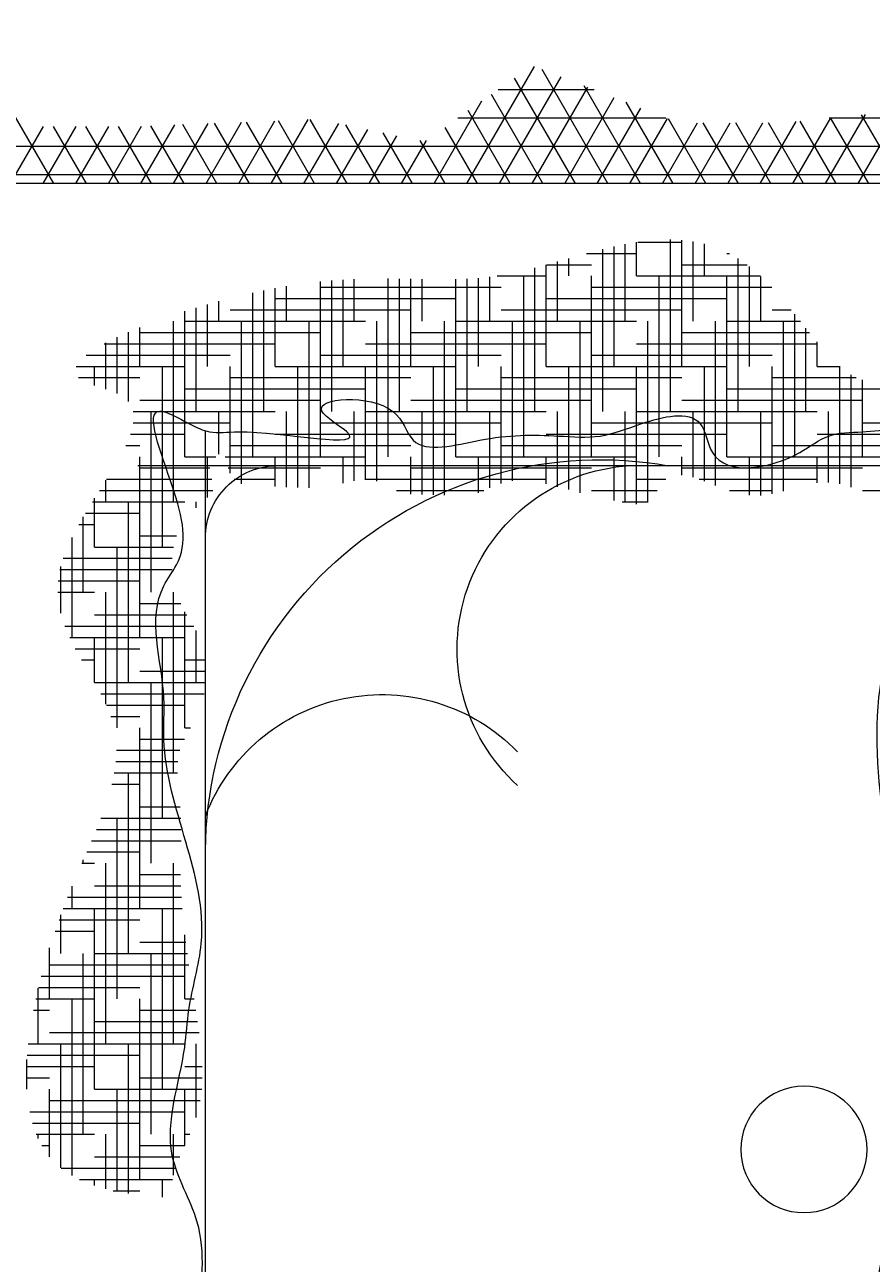
# Model space of a CAD drawing. Units: inches. Extents: x 3731 to 4318, y 1310 to 2388.
# Tile 18 of 57: x 4137 to 4176, y 1445 to 1502. Entities that reach past the tile are written whole.
import ezdxf

# ---------------------------------------------------------------- set-up
doc = ezdxf.new("R2010")
doc.units = ezdxf.units.IN
doc.layers.add('A-ANNO-DIMS', color=2, linetype='Continuous', lineweight=18)
doc.layers.add('A-FURN', color=8, linetype='Continuous', lineweight=13)
doc.styles.get("Standard").update_dxf_attribs({"font": 'arial.ttf'})
doc.dimstyles.get("Standard").update_dxf_attribs({"dimtxt": 0.18, "dimasz": 0.18, "dimexe": 0.18, "dimexo": 0.0625, "dimgap": 0.09, "dimtad": 0, "dimtih": 1, "dimtoh": 1, "dimdec": 4, "dimzin": 0, "dimdsep": 46, "dimtxsty": 'Standard', "dimcen": 0.09, "dimadec": 0, "dimazin": 0, "dimtfac": 1, "dimtdec": 4, "dimtofl": 0, "dimtmove": 0, "dimatfit": 3, "dimfxl": 1, "dimtolj": 1, "dimtzin": 0, "dimarcsym": 0})

# ---------------------------------------------------------------- blocks, each defined once
blk = doc.blocks.new('A$C200C7901')
for p, q in [((2.3121, 1.6596), (2.3121, 0.0201)), ((2, 0.2957), (2, 1.2957)), ((2.0224, 0.9977), (2.0224, 1.1977)), ((2.0224, 0.9977), (2.0224, 1.1977)), ((1.9974, 0.5977), (1.9974, 0.7977)), ((1.9974, 0.5977), (1.9974, 0.7977)), ((2.0724, 0.5977), (2.0724, 0.7977)), ((2.0724, 0.5977), (2.0724, 0.7977)), ((2.1474, 0.5977), (2.1474, 0.7977)), ((2.1474, 0.5977), (2.1474, 0.7977)), ((1.9849, 0.5477), (1.9849, 0.7477)), ((1.9849, 0.5477), (1.9849, 0.7477)), ((2.0599, 0.5477), (2.0599, 0.7477)), ((2.0599, 0.5477), (2.0599, 0.7477)), ((2.1349, 0.5477), (2.1349, 0.7477)), ((2.1349, 0.5477), (2.1349, 0.7477)), ((0.4061, 0.3703), (2.0386, 0.3703))]:
    blk.add_line(p, q)
at = {"linetype": 'ByBlock'}
for p, q in [((2.3224, 0.0468), (2.3224, 1.6627)), ((2.3224, 0.0468), (2.3224, 1.6627)), ((2.3537, 0.0056), (2.3537, 1.634)), ((2.3537, 0.0056), (2.3537, 1.634)), ((1.9724, 1.0977), (1.9724, 1.2927)), ((1.9724, 1.0977), (1.9724, 1.2927)), ((2.0474, 1.0977), (2.0474, 1.2977)), ((2.0474, 1.0977), (2.0474, 1.2977)), ((2.3849, 1.0607), (2.3849, 1.3013)), ((2.3849, 1.0607), (2.3849, 1.3013)), ((2.0349, 1.0477), (2.0349, 1.2477)), ((2.0349, 1.0477), (2.0349, 1.2477)), ((2.0099, 0.9477), (2.0099, 1.1477)), ((2.0099, 0.9477), (2.0099, 1.1477)), ((2.0849, 0.9477), (2.0849, 1.1477)), ((2.0849, 0.9477), (2.0849, 1.1477)), ((2.3121, 1.1408), (2.3884, 1.0967)), ((2.3121, 1.1408), (2.3884, 1.0967)), ((2.3121, 1.0928), (2.3915, 1.1386)), ((2.3121, 1.0928), (2.3915, 1.1386)), ((1.9974, 0.8977), (1.9974, 1.0977)), ((1.9974, 0.8977), (1.9974, 1.0977)), ((2.0099, 1.0977), (2.095, 1.0977)), ((2.0099, 1.0977), (2.095, 1.0977)), ((2.0724, 0.8977), (2.0724, 1.0977)), ((2.0724, 0.8977), (2.0724, 1.0977)), ((2.3121, 1.1047), (2.3851, 1.0625)), ((2.3121, 1.1047), (2.3851, 1.0625)), ((2.3121, 1.0567), (2.3887, 1.1009)), ((2.3121, 1.0567), (2.3887, 1.1009)), ((1.9763, 1.0852), (2.1005, 1.0852)), ((1.9763, 1.0852), (2.1005, 1.0852)), ((2.0974, 0.9977), (2.0974, 1.0909)), ((2.0974, 0.9977), (2.0974, 1.0909)), ((1.9799, 1.0727), (2.1099, 1.0727)), ((1.9799, 1.0727), (2.1099, 1.0727)), ((2.1099, 1.0477), (2.1099, 1.0729)), ((2.1099, 1.0477), (2.1099, 1.0729)), ((1.9815, 1.0602), (2.0599, 1.0602)), ((1.9815, 1.0602), (2.0599, 1.0602)), ((2.3121, 1.0686), (2.3813, 1.0286)), ((2.3121, 1.0686), (2.3813, 1.0286)), ((2.3121, 1.0206), (2.3851, 1.0628)), ((2.3121, 1.0206), (2.3851, 1.0628)), ((1.981, 1.0477), (2.0099, 1.0477)), ((1.981, 1.0477), (2.0099, 1.0477)), ((1.9849, 0.9171), (1.9849, 1.0477)), ((1.9849, 0.9171), (1.9849, 1.0477)), ((2.0599, 0.8477), (2.0599, 1.0477)), ((2.0599, 0.8477), (2.0599, 1.0477)), ((2.1099, 1.0477), (2.137, 1.0477)), ((2.1099, 1.0477), (2.137, 1.0477)), ((2.1349, 0.8477), (2.1349, 1.0477)), ((2.1349, 0.8477), (2.1349, 1.0477)), ((2.0599, 1.0352), (2.1523, 1.0352)), ((2.0599, 1.0352), (2.1523, 1.0352)), ((2.1474, 0.8977), (2.1474, 1.0391)), ((2.1474, 0.8977), (2.1474, 1.0391)), ((2.1599, 0.9477), (2.1599, 1.029)), ((2.1599, 0.9477), (2.1599, 1.029)), ((2.3121, 1.0325), (2.3795, 0.9936)), ((2.3121, 1.0325), (2.3795, 0.9936)), ((2.0099, 1.0227), (2.1678, 1.0227)), ((2.0099, 1.0227), (2.1678, 1.0227)), ((2.1724, 0.9977), (2.1724, 1.0189)), ((2.1724, 0.9977), (2.1724, 1.0189)), ((2.3121, 0.9846), (2.3809, 1.0242)), ((2.3121, 0.9846), (2.3809, 1.0242)), ((1.9718, 1.0102), (2.1599, 1.0102)), ((1.9718, 1.0102), (2.1599, 1.0102)), ((1.9688, 0.9977), (2.1099, 0.9977)), ((1.9688, 0.9977), (2.1099, 0.9977)), ((1.9724, 0.9504), (1.9724, 0.9977)), ((1.9724, 0.9504), (1.9724, 0.9977)), ((2.0474, 0.7977), (2.0474, 0.9977)), ((2.0474, 0.7977), (2.0474, 0.9977)), ((2.1224, 0.7977), (2.1224, 0.9977)), ((2.1224, 0.7977), (2.1224, 0.9977)), ((2.1974, 0.7977), (2.1974, 0.9972)), ((2.1974, 0.7977), (2.1974, 0.9972)), ((2.3121, 0.9964), (2.3795, 0.9575)), ((2.3121, 0.9964), (2.3795, 0.9575)), ((2.3121, 0.9485), (2.3795, 0.9874)), ((2.3121, 0.9485), (2.3795, 0.9874)), ((1.9671, 0.9852), (2.0599, 0.9852)), ((1.9671, 0.9852), (2.0599, 0.9852)), ((2.1599, 0.9852), (2.2095, 0.9852)), ((2.1599, 0.9852), (2.2095, 0.9852)), ((2.2099, 0.8477), (2.2099, 0.9848)), ((2.2099, 0.8477), (2.2099, 0.9848)), ((1.9672, 0.9727), (2.0099, 0.9727)), ((1.9672, 0.9727), (2.0099, 0.9727)), ((2.0599, 0.9602), (2.2294, 0.9602)), ((2.0599, 0.9602), (2.2294, 0.9602)), ((2.1099, 0.9727), (2.2204, 0.9727)), ((2.1099, 0.9727), (2.2204, 0.9727)), ((2.2224, 0.8977), (2.2224, 0.9702)), ((2.2224, 0.8977), (2.2224, 0.9702)), ((2.3121, 0.9603), (2.3795, 0.9215)), ((2.3121, 0.9603), (2.3795, 0.9215)), ((2.0099, 0.9477), (2.2099, 0.9477)), ((2.0099, 0.9477), (2.2099, 0.9477)), ((2.0349, 0.7477), (2.0349, 0.9477)), ((2.0349, 0.7477), (2.0349, 0.9477)), ((2.1099, 0.7477), (2.1099, 0.9477)), ((2.1099, 0.7477), (2.1099, 0.9477)), ((2.1849, 0.7477), (2.1849, 0.9477)), ((2.1849, 0.7477), (2.1849, 0.9477)), ((2.2349, 0.9477), (2.2349, 0.9506)), ((2.2349, 0.9477), (2.2349, 0.9506)), ((2.3121, 0.9124), (2.3795, 0.9513)), ((2.3121, 0.9124), (2.3795, 0.9513)), ((1.9781, 0.9352), (2.1599, 0.9352)), ((1.9781, 0.9352), (2.1599, 0.9352)), ((1.9829, 0.9227), (2.1099, 0.9227)), ((1.9829, 0.9227), (2.1099, 0.9227)), ((2.2099, 0.9227), (2.2455, 0.9227)), ((2.2099, 0.9227), (2.2455, 0.9227)), ((2.3121, 0.9243), (2.3838, 0.8829)), ((2.3121, 0.9243), (2.3838, 0.8829)), ((1.9871, 0.9102), (2.0599, 0.9102)), ((1.9871, 0.9102), (2.0599, 0.9102)), ((2.1599, 0.9102), (2.2481, 0.9102)), ((2.1599, 0.9102), (2.2481, 0.9102)), ((2.3121, 0.8763), (2.3795, 0.9152)), ((2.3121, 0.8763), (2.3795, 0.9152)), ((1.9894, 0.8977), (2.0099, 0.8977)), ((1.9894, 0.8977), (2.0099, 0.8977)), ((2.0224, 0.6977), (2.0224, 0.8977)), ((2.0224, 0.6977), (2.0224, 0.8977)), ((2.0974, 0.6977), (2.0974, 0.8977)), ((2.0974, 0.6977), (2.0974, 0.8977)), ((2.1099, 0.8977), (2.2496, 0.8977)), ((2.1099, 0.8977), (2.2496, 0.8977)), ((2.1724, 0.6977), (2.1724, 0.8977)), ((2.1724, 0.6977), (2.1724, 0.8977)), ((2.2474, 0.8489), (2.2474, 0.8977)), ((2.2474, 0.8489), (2.2474, 0.8977)), ((1.9849, 0.8477), (1.9849, 0.88)), ((1.9849, 0.8477), (1.9849, 0.88)), ((2.0599, 0.8852), (2.2501, 0.8852)), ((2.0599, 0.8852), (2.2501, 0.8852)), ((2.3121, 0.8882), (2.4022, 0.8362)), ((2.3121, 0.8882), (2.4022, 0.8362)), ((2.3121, 0.8402), (2.3842, 0.8818)), ((2.3121, 0.8402), (2.3842, 0.8818)), ((2.3849, 0.6497), (2.3849, 0.8801)), ((2.3849, 0.6497), (2.3849, 0.8801)), ((1.9724, 0.7977), (1.9724, 0.8703)), ((1.9724, 0.7977), (1.9724, 0.8703)), ((2.0099, 0.8727), (2.2099, 0.8727)), ((2.0099, 0.8727), (2.2099, 0.8727)), ((1.9599, 0.8317), (1.9599, 0.8604)), ((1.9599, 0.8317), (1.9599, 0.8604)), ((1.9599, 0.8602), (2.1599, 0.8602)), ((1.9599, 0.8602), (2.1599, 0.8602)), ((2.3121, 0.8041), (2.3958, 0.8524)), ((2.3121, 0.8041), (2.3958, 0.8524)), ((2.3121, 0.8521), (2.4205, 0.7895)), ((2.3121, 0.8521), (2.4205, 0.7895)), ((1.9574, 0.8477), (2.1099, 0.8477)), ((1.9574, 0.8477), (2.1099, 0.8477)), ((2.0099, 0.6477), (2.0099, 0.8477)), ((2.0099, 0.6477), (2.0099, 0.8477)), ((2.0849, 0.6477), (2.0849, 0.8477)), ((2.0849, 0.6477), (2.0849, 0.8477)), ((2.1599, 0.6477), (2.1599, 0.8477)), ((2.1599, 0.6477), (2.1599, 0.8477)), ((2.2099, 0.8477), (2.2472, 0.8477)), ((2.2099, 0.8477), (2.2472, 0.8477)), ((2.2349, 0.7923), (2.2349, 0.8477)), ((2.2349, 0.7923), (2.2349, 0.8477)), ((1.9593, 0.8352), (2.0599, 0.8352)), ((1.9593, 0.8352), (2.0599, 0.8352)), ((1.9615, 0.8227), (2.0099, 0.8227)), ((1.9615, 0.8227), (2.0099, 0.8227)), ((2.1099, 0.8227), (2.2425, 0.8227)), ((2.1099, 0.8227), (2.2425, 0.8227)), ((2.1599, 0.8352), (2.2451, 0.8352)), ((2.1599, 0.8352), (2.2451, 0.8352)), ((2.3121, 0.7681), (2.4073, 0.823)), ((2.3121, 0.7681), (2.4073, 0.823)), ((2.0599, 0.8102), (2.2396, 0.8102)), ((2.0599, 0.8102), (2.2396, 0.8102)), ((2.3121, 0.816), (2.4384, 0.7431)), ((2.3121, 0.816), (2.4384, 0.7431)), ((2.0099, 0.7977), (2.2099, 0.7977)), ((2.0099, 0.7977), (2.2099, 0.7977)), ((2.2224, 0.7483), (2.2224, 0.7977)), ((2.2224, 0.7483), (2.2224, 0.7977)), ((2.4162, 0.6946), (2.4162, 0.8006)), ((2.4162, 0.6946), (2.4162, 0.8006)), ((1.9699, 0.7852), (2.1599, 0.7852)), ((1.9699, 0.7852), (2.1599, 0.7852)), ((2.3121, 0.732), (2.4189, 0.7936)), ((2.3121, 0.732), (2.4189, 0.7936)), ((1.9734, 0.7727), (2.1099, 0.7727)), ((1.9734, 0.7727), (2.1099, 0.7727)), ((2.2099, 0.7727), (2.2294, 0.7727)), ((2.2099, 0.7727), (2.2294, 0.7727)), ((2.3121, 0.7799), (2.4287, 0.7126)), ((2.3121, 0.7799), (2.4287, 0.7126)), ((1.9767, 0.7602), (2.0599, 0.7602)), ((1.9767, 0.7602), (2.0599, 0.7602)), ((2.1599, 0.7602), (2.2258, 0.7602)), ((2.1599, 0.7602), (2.2258, 0.7602)), ((2.3121, 0.6959), (2.4303, 0.7641)), ((2.3121, 0.6959), (2.4303, 0.7641)), ((1.9797, 0.7477), (2.0099, 0.7477)), ((1.9797, 0.7477), (2.0099, 0.7477)), ((2.1099, 0.7477), (2.2222, 0.7477)), ((2.1099, 0.7477), (2.2222, 0.7477)), ((2.2099, 0.6933), (2.2099, 0.7477)), ((2.2099, 0.6933), (2.2099, 0.7477)), ((2.3121, 0.7438), (2.4108, 0.6869)), ((2.3121, 0.7438), (2.4108, 0.6869)), ((2.0599, 0.7352), (2.2188, 0.7352)), ((2.0599, 0.7352), (2.2188, 0.7352)), ((2.3121, 0.6598), (2.4417, 0.7346)), ((2.3121, 0.6598), (2.4417, 0.7346)), ((2.0099, 0.7227), (2.2099, 0.7227)), ((2.0099, 0.7227), (2.2099, 0.7227)), ((1.9831, 0.7102), (2.1599, 0.7102)), ((1.9831, 0.7102), (2.1599, 0.7102)), ((2.3121, 0.7078), (2.3929, 0.6611)), ((2.3121, 0.7078), (2.3929, 0.6611)), ((1.9804, 0.6977), (2.1099, 0.6977)), ((1.9804, 0.6977), (2.1099, 0.6977)), ((2.0474, 0.4977), (2.0474, 0.6977)), ((2.0474, 0.4977), (2.0474, 0.6977)), ((2.1224, 0.4977), (2.1224, 0.6977)), ((2.1224, 0.4977), (2.1224, 0.6977)), ((2.1974, 0.4977), (2.1974, 0.6977)), ((2.1974, 0.4977), (2.1974, 0.6977)), ((2.2099, 0.6977), (2.2106, 0.6977)), ((2.2099, 0.6977), (2.2106, 0.6977)), ((1.97, 0.6727), (2.0099, 0.6727)), ((1.97, 0.6727), (2.0099, 0.6727)), ((1.9724, 0.5818), (1.9724, 0.6786)), ((1.9724, 0.5818), (1.9724, 0.6786)), ((1.9753, 0.6852), (2.0599, 0.6852)), ((1.9753, 0.6852), (2.0599, 0.6852)), ((2.1099, 0.6727), (2.2075, 0.6727)), ((2.1099, 0.6727), (2.2075, 0.6727)), ((2.1599, 0.6852), (2.2088, 0.6852)), ((2.1599, 0.6852), (2.2088, 0.6852)), ((2.3121, 0.6237), (2.4036, 0.6765)), ((2.3121, 0.6237), (2.4036, 0.6765)), ((2.3121, 0.6717), (2.3744, 0.6357)), ((2.3121, 0.6717), (2.3744, 0.6357)), ((2.0599, 0.6602), (2.2067, 0.6602)), ((2.0599, 0.6602), (2.2067, 0.6602)), ((2.0099, 0.6477), (2.2062, 0.6477)), ((2.0099, 0.6477), (2.2062, 0.6477)), ((2.0349, 0.4477), (2.0349, 0.6477)), ((2.0349, 0.4477), (2.0349, 0.6477)), ((2.1099, 0.4477), (2.1099, 0.6477)), ((2.1099, 0.4477), (2.1099, 0.6477)), ((2.1849, 0.4477), (2.1849, 0.6477)), ((2.1849, 0.4477), (2.1849, 0.6477)), ((1.9673, 0.6352), (2.1599, 0.6352)), ((1.9673, 0.6352), (2.1599, 0.6352)), ((2.3121, 0.6356), (2.3598, 0.6081)), ((2.3121, 0.6356), (2.3598, 0.6081)), ((1.9678, 0.6227), (2.1099, 0.6227)), ((1.9678, 0.6227), (2.1099, 0.6227)), ((1.9679, 0.6102), (2.0599, 0.6102)), ((1.9679, 0.6102), (2.0599, 0.6102)), ((2.1599, 0.6102), (2.2064, 0.6102)), ((2.1599, 0.6102), (2.2064, 0.6102)), ((2.3121, 0.5876), (2.3598, 0.6151)), ((2.3121, 0.5876), (2.3598, 0.6151)), ((1.9685, 0.5977), (2.0099, 0.5977)), ((1.9685, 0.5977), (2.0099, 0.5977)), ((2.0224, 0.3977), (2.0224, 0.5977)), ((2.0224, 0.3977), (2.0224, 0.5977)), ((2.0974, 0.3977), (2.0974, 0.5977)), ((2.0974, 0.3977), (2.0974, 0.5977)), ((2.1099, 0.5977), (2.2066, 0.5977)), ((2.1099, 0.5977), (2.2066, 0.5977)), ((2.1724, 0.3977), (2.1724, 0.5977)), ((2.1724, 0.3977), (2.1724, 0.5977)), ((2.3121, 0.5995), (2.3682, 0.5671)), ((2.3121, 0.5995), (2.3682, 0.5671)), ((2.0599, 0.5852), (2.2069, 0.5852)), ((2.0599, 0.5852), (2.2069, 0.5852)), ((2.3121, 0.5515), (2.365, 0.5821)), ((2.3121, 0.5515), (2.365, 0.5821)), ((2.0099, 0.5727), (2.207, 0.5727)), ((2.0099, 0.5727), (2.207, 0.5727)), ((2.3121, 0.5634), (2.3771, 0.5259)), ((2.3121, 0.5634), (2.3771, 0.5259)), ((1.9827, 0.5602), (2.1599, 0.5602)), ((1.9827, 0.5602), (2.1599, 0.5602)), ((2.3121, 0.5155), (2.3719, 0.55)), ((2.3121, 0.5155), (2.3719, 0.55)), ((1.9831, 0.5352), (2.0599, 0.5352)), ((1.9831, 0.5352), (2.0599, 0.5352)), ((1.9842, 0.5477), (2.1099, 0.5477)), ((1.9842, 0.5477), (2.1099, 0.5477)), ((2.0099, 0.3923), (2.0099, 0.5477)), ((2.0099, 0.3923), (2.0099, 0.5477)), ((2.0849, 0.3477), (2.0849, 0.5477)), ((2.0849, 0.3477), (2.0849, 0.5477)), ((2.1599, 0.3477), (2.1599, 0.5477)), ((2.1599, 0.3477), (2.1599, 0.5477)), ((2.1599, 0.5352), (2.2065, 0.5352)), ((2.1599, 0.5352), (2.2065, 0.5352)), ((1.9807, 0.5227), (2.0099, 0.5227)), ((1.9807, 0.5227), (2.0099, 0.5227)), ((2.1099, 0.5227), (2.2058, 0.5227)), ((2.1099, 0.5227), (2.2058, 0.5227)), ((2.3121, 0.5273), (2.383, 0.4864)), ((2.3121, 0.5273), (2.383, 0.4864)), ((2.0599, 0.5102), (2.2049, 0.5102)), ((2.0599, 0.5102), (2.2049, 0.5102)), ((2.3121, 0.4794), (2.3788, 0.5179)), ((2.3121, 0.4794), (2.3788, 0.5179)), ((1.9974, 0.3957), (1.9974, 0.4977)), ((1.9974, 0.3957), (1.9974, 0.4977)), ((2.0099, 0.4977), (2.2038, 0.4977)), ((2.0099, 0.4977), (2.2038, 0.4977)), ((2.0724, 0.2977), (2.0724, 0.4977)), ((2.0724, 0.2977), (2.0724, 0.4977)), ((2.1474, 0.2977), (2.1474, 0.4977)), ((2.1474, 0.2977), (2.1474, 0.4977)), ((1.9755, 0.4852), (2.1599, 0.4852)), ((1.9755, 0.4852), (2.1599, 0.4852)), ((2.3121, 0.4912), (2.3817, 0.4511)), ((2.3121, 0.4912), (2.3817, 0.4511)), ((2.3121, 0.4433), (2.383, 0.4842)), ((2.3121, 0.4433), (2.383, 0.4842)), ((1.9757, 0.4727), (2.1099, 0.4727)), ((1.9757, 0.4727), (2.1099, 0.4727)), ((1.9762, 0.4602), (2.0599, 0.4602)), ((1.9762, 0.4602), (2.0599, 0.4602)), ((2.1599, 0.4602), (2.1987, 0.4602)), ((2.1599, 0.4602), (2.1987, 0.4602)), ((2.3121, 0.4552), (2.3803, 0.4158)), ((2.3121, 0.4552), (2.3803, 0.4158)), ((1.9768, 0.4477), (2.0099, 0.4477)), ((1.9768, 0.4477), (2.0099, 0.4477)), ((1.9849, 0.402), (1.9849, 0.4477)), ((1.9849, 0.402), (1.9849, 0.4477)), ((2.0599, 0.2903), (2.0599, 0.4477)), ((2.0599, 0.2903), (2.0599, 0.4477)), ((2.1099, 0.4477), (2.1965, 0.4477)), ((2.1099, 0.4477), (2.1965, 0.4477)), ((2.1349, 0.2582), (2.1349, 0.4477)), ((2.1349, 0.2582), (2.1349, 0.4477)), ((2.3121, 0.4072), (2.3815, 0.4473)), ((2.3121, 0.4072), (2.3815, 0.4473)), ((2.0599, 0.4352), (2.194, 0.4352)), ((2.0599, 0.4352), (2.194, 0.4352)), ((2.0099, 0.4227), (2.1913, 0.4227)), ((2.0099, 0.4227), (2.1913, 0.4227)), ((2.3121, 0.4191), (2.3789, 0.3805)), ((2.3121, 0.4191), (2.3789, 0.3805)), ((1.9797, 0.4102), (2.1599, 0.4102)), ((1.9797, 0.4102), (2.1599, 0.4102)), ((1.9915, 0.3977), (2.1099, 0.3977)), ((1.9915, 0.3977), (2.1099, 0.3977)), ((2.0474, 0.2905), (2.0474, 0.3977)), ((2.0474, 0.2905), (2.0474, 0.3977)), ((2.1224, 0.2385), (2.1224, 0.3977)), ((2.1224, 0.2385), (2.1224, 0.3977)), ((2.3121, 0.3711), (2.3801, 0.4103)), ((2.3121, 0.3711), (2.3801, 0.4103)), ((2.0127, 0.3852), (2.0599, 0.3852)), ((2.0127, 0.3852), (2.0599, 0.3852)), ((2.1599, 0.3852), (2.1819, 0.3852)), ((2.1599, 0.3852), (2.1819, 0.3852)), ((1.7599, 0.2477), (1.7599, 0.3703)), ((1.7599, 0.2477), (1.7599, 0.3703)), ((1.7724, 0.2977), (1.7724, 0.3703)), ((1.7724, 0.2977), (1.7724, 0.3703)), ((1.7849, 0.3477), (1.7849, 0.3703)), ((1.7849, 0.3477), (1.7849, 0.3703)), ((1.9648, 0.3727), (2.0099, 0.3727)), ((1.9648, 0.3727), (2.0099, 0.3727)), ((1.9724, 0.253), (1.9724, 0.3785)), ((1.9724, 0.253), (1.9724, 0.3785)), ((1.9849, 0.2609), (1.9849, 0.3774)), ((1.9849, 0.2609), (1.9849, 0.3774)), ((1.9974, 0.2977), (1.9974, 0.3753)), ((1.9974, 0.2977), (1.9974, 0.3753)), ((2.0099, 0.3477), (2.0099, 0.382)), ((2.0099, 0.3477), (2.0099, 0.382)), ((2.1099, 0.3727), (2.1784, 0.3727)), ((2.1099, 0.3727), (2.1784, 0.3727)), ((2.3121, 0.383), (2.3775, 0.3452)), ((2.3121, 0.383), (2.3775, 0.3452)), ((2.3121, 0.335), (2.3786, 0.3734)), ((2.3121, 0.335), (2.3786, 0.3734)), ((1.2785, 0.3602), (1.3599, 0.3602)), ((1.2785, 0.3602), (1.3599, 0.3602)), ((1.2974, 0.1977), (1.2974, 0.3647)), ((1.2974, 0.1977), (1.2974, 0.3647)), ((1.3099, 0.2477), (1.3099, 0.3663)), ((1.3099, 0.2477), (1.3099, 0.3663)), ((1.3224, 0.2977), (1.3224, 0.3669)), ((1.3224, 0.2977), (1.3224, 0.3669)), ((1.3349, 0.3477), (1.3349, 0.3668)), ((1.3349, 0.3477), (1.3349, 0.3668)), ((1.3724, 0.1977), (1.3724, 0.3634)), ((1.3724, 0.1977), (1.3724, 0.3634)), ((1.3849, 0.2477), (1.3849, 0.3616)), ((1.3849, 0.2477), (1.3849, 0.3616)), ((1.3974, 0.2977), (1.3974, 0.3597)), ((1.3974, 0.2977), (1.3974, 0.3597)), ((1.4099, 0.3477), (1.4099, 0.3578)), ((1.4099, 0.3477), (1.4099, 0.3578)), ((1.7474, 0.2546), (1.7474, 0.3689)), ((1.7474, 0.2546), (1.7474, 0.3689)), ((1.7599, 0.3602), (1.8177, 0.3602)), ((1.7599, 0.3602), (1.8177, 0.3602)), ((1.8224, 0.2148), (1.8224, 0.3575)), ((1.8224, 0.2148), (1.8224, 0.3575)), ((1.9532, 0.3602), (1.9599, 0.3602)), ((1.9532, 0.3602), (1.9599, 0.3602)), ((2.0599, 0.3602), (2.1747, 0.3602)), ((2.0599, 0.3602), (2.1747, 0.3602)), ((1.2474, 0.2977), (1.2474, 0.3476)), ((1.2474, 0.2977), (1.2474, 0.3476)), ((1.2475, 0.3477), (1.3099, 0.3477)), ((1.2475, 0.3477), (1.3099, 0.3477)), ((1.2599, 0.3477), (1.2599, 0.3531)), ((1.2599, 0.3477), (1.2599, 0.3531)), ((1.2849, 0.1758), (1.2849, 0.3477)), ((1.2849, 0.1758), (1.2849, 0.3477)), ((1.3599, 0.1741), (1.3599, 0.3477)), ((1.3599, 0.1741), (1.3599, 0.3477)), ((1.4099, 0.3477), (1.4806, 0.3477)), ((1.4099, 0.3477), (1.4806, 0.3477)), ((1.4349, 0.1886), (1.4349, 0.3477)), ((1.4349, 0.1886), (1.4349, 0.3477)), ((1.4474, 0.1977), (1.4474, 0.3521)), ((1.4474, 0.1977), (1.4474, 0.3521)), ((1.4599, 0.2477), (1.4599, 0.3504)), ((1.4599, 0.2477), (1.4599, 0.3504)), ((1.4724, 0.2977), (1.4724, 0.3487)), ((1.4724, 0.2977), (1.4724, 0.3487)), ((1.5099, 0.2129), (1.5099, 0.3447)), ((1.5099, 0.2129), (1.5099, 0.3447)), ((1.5224, 0.2177), (1.5224, 0.3438)), ((1.5224, 0.2177), (1.5224, 0.3438)), ((1.5349, 0.2477), (1.5349, 0.3431)), ((1.5349, 0.2477), (1.5349, 0.3431)), ((1.5474, 0.2977), (1.5474, 0.3428)), ((1.5474, 0.2977), (1.5474, 0.3428)), ((1.5849, 0.2443), (1.5849, 0.3434)), ((1.5849, 0.2443), (1.5849, 0.3434)), ((1.5974, 0.2496), (1.5974, 0.3435)), ((1.5974, 0.2496), (1.5974, 0.3435)), ((1.6099, 0.2546), (1.6099, 0.3432)), ((1.6099, 0.2546), (1.6099, 0.3432)), ((1.6974, 0.2977), (1.6974, 0.3472)), ((1.6974, 0.2977), (1.6974, 0.3472)), ((1.7099, 0.3477), (1.7099, 0.3539)), ((1.7099, 0.3477), (1.7099, 0.3539)), ((1.7099, 0.3477), (1.8383, 0.3477)), ((1.7099, 0.3477), (1.8383, 0.3477)), ((1.7349, 0.2607), (1.7349, 0.3477)), ((1.7349, 0.2607), (1.7349, 0.3477)), ((1.8099, 0.2201), (1.8099, 0.3477)), ((1.8099, 0.2201), (1.8099, 0.3477)), ((1.8349, 0.2477), (1.8349, 0.3497)), ((1.8349, 0.2477), (1.8349, 0.3497)), ((1.8474, 0.2977), (1.8474, 0.3432)), ((1.8474, 0.2977), (1.8474, 0.3432)), ((1.9599, 0.2452), (1.9599, 0.3477)), ((1.9599, 0.2452), (1.9599, 0.3477)), ((2.0099, 0.3477), (2.1708, 0.3477)), ((2.0099, 0.3477), (2.1708, 0.3477)), ((2.0349, 0.2874), (2.0349, 0.3477)), ((2.0349, 0.2874), (2.0349, 0.3477)), ((2.1099, 0.2274), (2.1099, 0.3477)), ((2.1099, 0.2274), (2.1099, 0.3477)), ((2.3121, 0.3469), (2.3761, 0.31)), ((2.3121, 0.3469), (2.3761, 0.31)), ((1.2099, 0.2308), (1.2099, 0.334)), ((1.2099, 0.2308), (1.2099, 0.334)), ((1.2148, 0.3352), (1.2599, 0.3352)), ((1.2148, 0.3352), (1.2599, 0.3352)), ((1.2224, 0.2106), (1.2224, 0.3375)), ((1.2224, 0.2106), (1.2224, 0.3375)), ((1.2349, 0.2477), (1.2349, 0.3422)), ((1.2349, 0.2477), (1.2349, 0.3422)), ((1.3599, 0.3352), (1.5599, 0.3352)), ((1.3599, 0.3352), (1.5599, 0.3352)), ((1.6224, 0.2977), (1.6224, 0.3424)), ((1.6224, 0.2977), (1.6224, 0.3424)), ((1.6599, 0.2695), (1.6599, 0.3394)), ((1.6599, 0.2695), (1.6599, 0.3394)), ((1.6599, 0.3352), (1.8599, 0.3352)), ((1.6599, 0.3352), (1.8599, 0.3352)), ((1.6724, 0.2713), (1.6724, 0.3398)), ((1.6724, 0.2713), (1.6724, 0.3398)), ((1.6849, 0.272), (1.6849, 0.3422)), ((1.6849, 0.272), (1.6849, 0.3422)), ((1.8849, 0.2093), (1.8849, 0.3337)), ((1.8849, 0.2093), (1.8849, 0.3337)), ((1.8974, 0.2129), (1.8974, 0.3335)), ((1.8974, 0.2129), (1.8974, 0.3335)), ((1.9099, 0.2477), (1.9099, 0.3349)), ((1.9099, 0.2477), (1.9099, 0.3349)), ((1.9224, 0.2977), (1.9224, 0.3385)), ((1.9224, 0.2977), (1.9224, 0.3385)), ((1.9599, 0.3352), (2.1599, 0.3352)), ((1.9599, 0.3352), (2.1599, 0.3352)), ((2.3121, 0.299), (2.3772, 0.3365)), ((2.3121, 0.299), (2.3772, 0.3365)), ((1.1904, 0.3227), (1.2099, 0.3227)), ((1.1904, 0.3227), (1.2099, 0.3227)), ((1.3099, 0.3227), (1.5099, 0.3227)), ((1.3099, 0.3227), (1.5099, 0.3227)), ((1.6099, 0.3227), (1.8099, 0.3227)), ((1.6099, 0.3227), (1.8099, 0.3227)), ((1.9099, 0.3227), (2.1099, 0.3227)), ((1.9099, 0.3227), (2.1099, 0.3227)), ((1.2599, 0.3102), (1.4599, 0.3102)), ((1.2599, 0.3102), (1.4599, 0.3102)), ((1.5599, 0.3102), (1.7599, 0.3102)), ((1.5599, 0.3102), (1.7599, 0.3102)), ((1.8599, 0.3102), (2.0599, 0.3102)), ((1.8599, 0.3102), (2.0599, 0.3102)), ((2.3121, 0.3108), (2.3755, 0.2742)), ((2.3121, 0.3108), (2.3755, 0.2742)), ((1.1974, 0.2683), (1.1974, 0.2977)), ((1.1974, 0.2683), (1.1974, 0.2977)), ((1.2099, 0.2977), (1.4099, 0.2977)), ((1.2099, 0.2977), (1.4099, 0.2977)), ((1.2724, 0.1788), (1.2724, 0.2977)), ((1.2724, 0.1788), (1.2724, 0.2977)), ((1.3474, 0.173), (1.3474, 0.2977)), ((1.3474, 0.173), (1.3474, 0.2977)), ((1.4224, 0.1854), (1.4224, 0.2977)), ((1.4224, 0.1854), (1.4224, 0.2977)), ((1.4974, 0.2083), (1.4974, 0.2977)), ((1.4974, 0.2083), (1.4974, 0.2977)), ((1.5099, 0.2977), (1.7099, 0.2977)), ((1.5099, 0.2977), (1.7099, 0.2977)), ((1.5724, 0.2389), (1.5724, 0.2977)), ((1.5724, 0.2389), (1.5724, 0.2977)), ((1.6474, 0.2668), (1.6474, 0.2977)), ((1.6474, 0.2668), (1.6474, 0.2977)), ((1.7224, 0.2658), (1.7224, 0.2977)), ((1.7224, 0.2658), (1.7224, 0.2977)), ((1.7974, 0.2263), (1.7974, 0.2977)), ((1.7974, 0.2263), (1.7974, 0.2977)), ((1.8099, 0.2977), (2.0099, 0.2977)), ((1.8099, 0.2977), (2.0099, 0.2977)), ((1.8724, 0.2072), (1.8724, 0.2977)), ((1.8724, 0.2072), (1.8724, 0.2977)), ((1.9474, 0.2376), (1.9474, 0.2977)), ((1.9474, 0.2376), (1.9474, 0.2977)), ((2.0224, 0.2822), (2.0224, 0.2977)), ((2.0224, 0.2822), (2.0224, 0.2977)), ((2.0974, 0.2299), (2.0974, 0.2977)), ((2.0974, 0.2299), (2.0974, 0.2977)), ((2.1099, 0.2977), (2.153, 0.2977)), ((2.1099, 0.2977), (2.153, 0.2977)), ((2.3121, 0.2629), (2.3757, 0.2996)), ((2.3121, 0.2629), (2.3757, 0.2996)), ((1.1943, 0.2852), (1.3599, 0.2852)), ((1.1943, 0.2852), (1.3599, 0.2852)), ((1.4599, 0.2852), (1.6599, 0.2852)), ((1.4599, 0.2852), (1.6599, 0.2852)), ((1.7599, 0.2852), (1.9599, 0.2852)), ((1.7599, 0.2852), (1.9599, 0.2852)), ((2.0708, 0.2852), (2.1478, 0.2852)), ((2.0708, 0.2852), (2.1478, 0.2852)), ((2.3121, 0.2747), (2.3755, 0.2381)), ((2.3121, 0.2747), (2.3755, 0.2381)), ((1.1965, 0.2727), (1.3099, 0.2727)), ((1.1965, 0.2727), (1.3099, 0.2727)), ((1.4099, 0.2727), (1.6099, 0.2727)), ((1.4099, 0.2727), (1.6099, 0.2727)), ((1.7099, 0.2727), (1.9099, 0.2727)), ((1.7099, 0.2727), (1.9099, 0.2727)), ((2.08, 0.2727), (2.1422, 0.2727)), ((2.08, 0.2727), (2.1422, 0.2727)), ((2.3121, 0.2268), (2.3755, 0.2634)), ((2.3121, 0.2268), (2.3755, 0.2634)), ((1.1994, 0.2602), (1.2599, 0.2602)), ((1.1994, 0.2602), (1.2599, 0.2602)), ((1.2031, 0.2477), (1.2099, 0.2477)), ((1.2031, 0.2477), (1.2099, 0.2477)), ((1.2599, 0.1831), (1.2599, 0.2477)), ((1.2599, 0.1831), (1.2599, 0.2477)), ((1.3099, 0.2477), (1.5099, 0.2477)), ((1.3099, 0.2477), (1.5099, 0.2477)), ((1.3349, 0.1723), (1.3349, 0.2477)), ((1.3349, 0.1723), (1.3349, 0.2477)), ((1.3599, 0.2602), (1.5599, 0.2602)), ((1.3599, 0.2602), (1.5599, 0.2602)), ((1.4099, 0.1825), (1.4099, 0.2477)), ((1.4099, 0.1825), (1.4099, 0.2477)), ((1.4849, 0.2039), (1.4849, 0.2477)), ((1.4849, 0.2039), (1.4849, 0.2477)), ((1.5599, 0.2335), (1.5599, 0.2477)), ((1.5599, 0.2335), (1.5599, 0.2477)), ((1.7361, 0.2602), (1.8599, 0.2602)), ((1.7361, 0.2602), (1.8599, 0.2602)), ((1.7599, 0.2477), (1.8099, 0.2477)), ((1.7599, 0.2477), (1.8099, 0.2477)), ((1.7849, 0.2332), (1.7849, 0.2477)), ((1.7849, 0.2332), (1.7849, 0.2477)), ((1.8599, 0.2068), (1.8599, 0.2477)), ((1.8599, 0.2068), (1.8599, 0.2477)), ((1.9099, 0.2477), (1.9639, 0.2477)), ((1.9099, 0.2477), (1.9639, 0.2477)), ((1.9349, 0.2304), (1.9349, 0.2477)), ((1.9349, 0.2304), (1.9349, 0.2477)), ((1.9599, 0.2602), (1.9838, 0.2602)), ((1.9599, 0.2602), (1.9838, 0.2602)), ((2.0848, 0.2602), (2.1359, 0.2602)), ((2.0848, 0.2602), (2.1359, 0.2602)), ((2.0888, 0.2477), (2.1099, 0.2477)), ((2.0888, 0.2477), (2.1099, 0.2477)), ((1.2599, 0.2352), (1.4599, 0.2352)), ((1.2599, 0.2352), (1.4599, 0.2352)), ((1.5599, 0.2352), (1.5638, 0.2352)), ((1.5599, 0.2352), (1.5638, 0.2352)), ((1.8599, 0.2352), (1.9433, 0.2352)), ((1.8599, 0.2352), (1.9433, 0.2352)), ((2.3121, 0.2387), (2.3755, 0.202)), ((2.3121, 0.2387), (2.3755, 0.202)), ((1.2142, 0.2227), (1.4099, 0.2227)), ((1.2142, 0.2227), (1.4099, 0.2227)), ((1.5099, 0.2227), (1.5346, 0.2227)), ((1.5099, 0.2227), (1.5346, 0.2227)), ((1.8099, 0.2227), (1.9203, 0.2227)), ((1.8099, 0.2227), (1.9203, 0.2227)), ((2.3121, 0.1907), (2.3755, 0.2273)), ((2.3121, 0.1907), (2.3755, 0.2273)), ((1.2227, 0.2102), (1.3599, 0.2102)), ((1.2227, 0.2102), (1.3599, 0.2102)), ((1.4599, 0.2102), (1.5027, 0.2102)), ((1.4599, 0.2102), (1.5027, 0.2102)), ((1.8368, 0.2102), (1.8884, 0.2102)), ((1.8368, 0.2102), (1.8884, 0.2102)), ((1.2351, 0.1977), (1.3099, 0.1977)), ((1.2351, 0.1977), (1.3099, 0.1977)), ((1.2474, 0.1892), (1.2474, 0.1977)), ((1.2474, 0.1892), (1.2474, 0.1977)), ((1.3224, 0.1722), (1.3224, 0.1977)), ((1.3224, 0.1722), (1.3224, 0.1977)), ((1.3974, 0.1799), (1.3974, 0.1977)), ((1.3974, 0.1799), (1.3974, 0.1977)), ((1.4099, 0.1977), (1.4662, 0.1977)), ((1.4099, 0.1977), (1.4662, 0.1977)), ((2.3121, 0.2026), (2.3953, 0.1545)), ((2.3121, 0.2026), (2.3953, 0.1545)), ((1.2552, 0.1852), (1.2599, 0.1852)), ((1.2552, 0.1852), (1.2599, 0.1852)), ((1.3599, 0.1852), (1.4215, 0.1852)), ((1.3599, 0.1852), (1.4215, 0.1852)), ((2.3121, 0.1546), (2.3755, 0.1912)), ((2.3121, 0.1546), (2.3755, 0.1912)), ((1.3099, 0.1727), (1.3428, 0.1727)), ((1.3099, 0.1727), (1.3428, 0.1727))]:
    blk.add_line(p, q, dxfattribs=at)
blk.add_circle((1.2431, 1.0329), 0.0699)
for centre, radius, start, end in [((1.5693, 0.8075), 0.4372, 269.0679, 9.9322), ((1.7969, 0.8525), 0.2035, 222.1514, 356.4639), ((1.5372, 0.5659), 0.2094, 290.9415, 45.7647), ((1.92, 0.4503), 0.08, 270, 0)]:
    blk.add_arc(centre, radius, start, end)
blk.add_open_spline([(0.4856, 1.3429), (0.5504, 1.3182), (0.6715, 1.2721), (0.8374, 1.0498), (1.1164, 1.1183), (1.3878, 1.1816), (1.5888, 1.1102), (1.8403, 1.1127), (1.9415, 1.2178), (2.0032, 1.2819)], degree=3, knots=[0, 0, 0, 0, 205.411753, 383.654933, 772.067458, 921.644661, 1226.793228, 1388.983508, 1642.292305, 1642.292305, 1642.292305, 1642.292305])
blk.add_open_spline([(0.473, 1.2954), (0.4739, 1.2781), (0.4755, 1.2477), (0.5032, 1.2084), (0.4801, 1.1701), (0.4928, 1.1255), (0.4674, 1.0912), (0.4579, 1.0351), (0.501, 0.9724), (0.4311, 0.8832), (0.4902, 0.8637), (0.4843, 0.8288), (0.4774, 0.7906), (0.4625, 0.7457), (0.459, 0.6999), (0.4816, 0.6664), (0.4748, 0.625), (0.4791, 0.5889), (0.4533, 0.5528), (0.4738, 0.5004), (0.4658, 0.4502), (0.4696, 0.3946), (0.4189, 0.3935), (0.4493, 0.3684), (0.4694, 0.3857), (0.4922, 0.3576), (0.5297, 0.3262), (0.5917, 0.3353), (0.6454, 0.3754), (0.7083, 0.3741), (0.7643, 0.3328), (0.826, 0.346), (0.925, 0.3388), (1.0353, 0.3593), (1.1561, 0.3744), (1.2477, 0.3154), (1.3302, 0.3474), (1.4086, 0.3512), (1.5217, 0.3878), (1.6362, 0.3176), (1.7682, 0.3285), (1.8402, 0.3019), (1.9071, 0.3529), (1.9647, 0.3412), (2.0795, 0.2948), (2.0472, 0.3498), (2.0343, 0.3772), (2.0435, 0.43), (2.0109, 0.5782), (2.0746, 0.4643), (2.0805, 0.584), (2.0084, 0.5979), (2.0343, 0.6846), (2.0344, 0.746), (2.0293, 0.8096), (2.0489, 0.8545), (2.0652, 0.9218), (1.9842, 0.9297), (2.0007, 1.0162), (2.0367, 1.0585), (2.0367, 1.1102), (2.0457, 1.1647), (2.0226, 1.2084), (2.0234, 1.2306), (2.0236, 1.2352)], degree=3, knots=[0, 0, 0, 0, 51.660678, 90.967412, 128.902454, 170.303599, 219.852997, 247.834962, 336.321557, 429.35469, 458.821847, 477.222321, 524.135809, 581.038434, 617.839381, 657.146115, 693.947125, 740.178081, 760.753248, 820.731705, 885.133458, 928.777044, 953.563729, 976.574207, 995.553042, 1018.563482, 1064.584401, 1147.951297, 1174.787598, 1266.851571, 1308.018447, 1377.066427, 1441.511314, 1608.245014, 1714.11869, 1792.771707, 1913.247991, 1954.931389, 2029.864445, 2259.189419, 2305.221512, 2429.507982, 2456.344283, 2543.92595, 2627.925037, 2662.96218, 2687.736879, 2719.937755, 2839.540991, 2875.47895, 2953.681041, 2993.270313, 3066.872333, 3154.395764, 3200.397042, 3248.426375, 3312.828127, 3347.881398, 3444.484026, 3481.577522, 3518.665244, 3592.267265, 3644.719162, 3658.519501, 3658.519501, 3658.519501, 3658.519501], dxfattribs=at)
blk = doc.blocks.new('*D32')
at = {"layer": 'A-ANNO-DIMS', "color": 0, "lineweight": -2, "transparency": 16777216}
for p, q in [((4269.211, 1592.319), (4269.211, 1310.251)), ((3835.209, 1359.319), (3835.209, 1310.251)), ((3835.389, 1310.431), (4051.918, 1310.431)), ((4269.031, 1310.431), (4052.502, 1310.431))]:
    blk.add_line(p, q, dxfattribs=at)
at = {"layer": 'A-ANNO-DIMS', "color": 0, "transparency": 16777216}
for points in [[(3835.389, 1310.461), (3835.389, 1310.401), (3835.209, 1310.431)], [(4269.031, 1310.461), (4269.031, 1310.401), (4269.211, 1310.431)]]:
    blk.add_solid(points, dxfattribs=at)
at = {"layer": 'Defpoints', "color": 0, "transparency": 16777216}
for p in [(4269.211, 1592.382), (3835.209, 1359.382), (4269.211, 1310.431)]:
    blk.add_point(p, dxfattribs=at)
at = {"layer": 'A-ANNO-DIMS', "color": 0, "transparency": 16777216, "insert": (4052.21, 1310.431), "char_height": 0.18, "attachment_point": 5}
blk.add_mtext('\\A1;434', dxfattribs=at)
blk = doc.blocks.new('*D46')
at = {"layer": 'A-ANNO-DIMS', "color": 0, "lineweight": -2, "transparency": 16777216}
for p, q in [((4112.209, 1854.319), (4112.209, 1310.251)), ((4192.209, 1854.319), (4192.209, 1310.251)), ((4112.389, 1310.431), (4151.99, 1310.431)), ((4192.029, 1310.431), (4152.428, 1310.431))]:
    blk.add_line(p, q, dxfattribs=at)
at = {"layer": 'A-ANNO-DIMS', "color": 0, "transparency": 16777216}
for points in [[(4112.389, 1310.461), (4112.389, 1310.401), (4112.209, 1310.431)], [(4192.029, 1310.461), (4192.029, 1310.401), (4192.209, 1310.431)]]:
    blk.add_solid(points, dxfattribs=at)
at = {"layer": 'Defpoints', "color": 0, "transparency": 16777216}
for p in [(4112.209, 1854.382), (4192.209, 1854.382), (4192.209, 1310.431)]:
    blk.add_point(p, dxfattribs=at)
at = {"layer": 'A-ANNO-DIMS', "color": 0, "transparency": 16777216, "insert": (4152.209, 1310.431), "char_height": 0.18, "attachment_point": 5}
blk.add_mtext('\\A1;80', dxfattribs=at)

msp = doc.modelspace()

# ---------------------------------------------------------------- block references
at = {"layer": 'A-FURN', "xscale": -41.1071563136412, "yscale": 41.1071563136412, "zscale": 41.1071563136412, "rotation": 270}
msp.add_blockref('A$C200C7901', (4130.025, 1399.263), dxfattribs=at)

# ---------------------------------------------------------------- dimensions: what is measured, and where the dimension line sits
at = {"layer": 'A-ANNO-DIMS'}
for base, p1, p2, picture, middle in [((4192.209, 1310.431), (4112.209, 1854.382), (4192.209, 1854.382), '*D46', (4152.209, 1310.431)), ((4269.211, 1310.431), (3835.209, 1359.382), (4269.211, 1592.382), '*D32', (4052.21, 1310.431))]:
    dim = msp.add_linear_dim(base=base, p1=p1, p2=p2, dimstyle='Standard', override={"dimdec": 0, "dimlfac": 1, "dimrnd": 0, "dimzin": 0, "dimdsep": 46, "dimlunit": 2}, dxfattribs=at)
    dim.commit()
    dim.dimension.update_dxf_attribs({"geometry": picture, "text_midpoint": middle})

doc.saveas('drawing.dxf')
